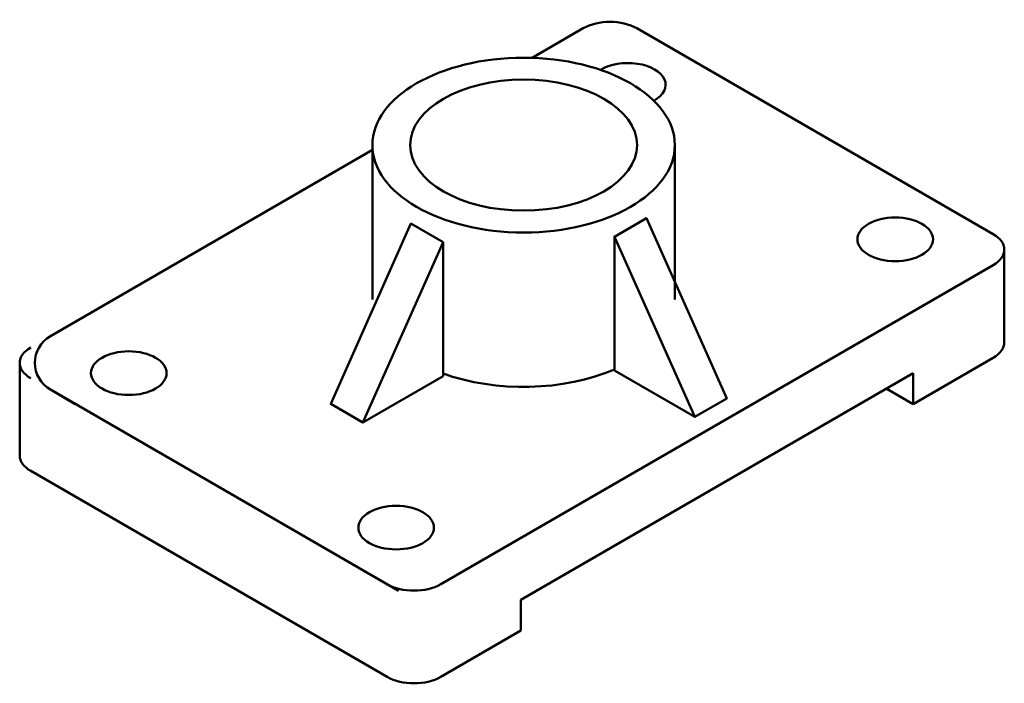
# Model space of a CAD drawing. Units: millimetres. Extents: x 2166 to 2644, y 1138 to 1460.
import ezdxf

# ---------------------------------------------------------------- set-up
doc = ezdxf.new("R2010")
doc.units = ezdxf.units.MM
doc.layers.add('M-OUTL', color=7, linetype='Continuous', lineweight=50)

msp = doc.modelspace()

# ---------------------------------------------------------------- linework, layer by layer
at = {"layer": 'M-OUTL'}
for p, q in [((2414.45, 1441.4), (2439.37, 1455.79)), ((2638.56, 1355.79), (2465.35, 1455.79)), ((2336.87, 1399.04), (2336.87, 1324.04)), ((2483.84, 1399.04), (2483.84, 1324.04)), ((2643.94, 1303.29), (2643.94, 1348.29)), ((2370.09, 1185.79), (2638.56, 1340.79)), ((2165.52, 1248.29), (2165.52, 1293.29)), ((2599.58, 1273.29), (2638.56, 1295.79)), ((2409.06, 1178.29), (2599.58, 1288.29)), ((2599.58, 1273.29), (2599.58, 1288.29)), ((2180.41, 1280.3), (2349.6, 1182.62)), ((2599.58, 1273.29), (2586.59, 1280.79)), ((2344.11, 1140.79), (2170.9, 1240.79)), ((2409.06, 1163.29), (2409.06, 1178.29)), ((2370.09, 1140.79), (2409.06, 1163.29))]:
    msp.add_line(p, q, dxfattribs=at)
msp.add_lwpolyline([(2336.98, 1396.68), (2180.41, 1306.28, 0.57735), (2180.41, 1280.3), (2192.55, 1273.29)], format="xyb", dxfattribs=at)
for points in [[(2493.49, 1267.04), (2509.08, 1276.04), (2470.11, 1363.54), (2454.52, 1354.54)], [(2332.25, 1264.39), (2316.66, 1273.39), (2355.63, 1360.89), (2371.22, 1351.89)]]:
    msp.add_lwpolyline(points, dxfattribs=at)
for points in [[(2454.52, 1289.54), (2493.49, 1267.04), (2454.52, 1354.54)], [(2371.22, 1286.89), (2332.25, 1264.39), (2371.22, 1351.89)]]:
    msp.add_lwpolyline(points, close=True, dxfattribs=at)
for centre, major_axis, start_param, end_param in [((2452.36, 1448.29), (-18.37, 0), 3.926991, 5.497787), ((2461.02, 1428.29), (-18.37, 0), 2.32895, 5.525032), ((2625.57, 1348.29), (18.37, 0), 0, 0.785398), ((2625.57, 1348.29), (18.37, 0), 5.497787, 6.283185), ((2625.57, 1303.29), (18.37, 0), 5.497787, 6.283185), ((2183.89, 1293.29), (-18.37, 0), 5.497787, 6.283185), ((2183.89, 1293.29), (-18.37, 0), 0, 0.785398), ((2410.36, 1324.04), (73.48, 0), 4.146433, 5.357192), ((2183.89, 1248.29), (-18.37, 0), 0, 0.785398), ((2357.1, 1193.29), (18.37, 0), 3.926991, 5.497787), ((2357.1, 1148.29), (18.37, 0), 3.926991, 5.497787)]:
    msp.add_ellipse(centre, major_axis=major_axis, ratio=0.57735, start_param=start_param, end_param=end_param, dxfattribs=at)
for centre, major_axis in [((2410.36, 1399.04), (-73.48, 0)), ((2410.36, 1399.04), (-55.11, 0)), ((2590.93, 1353.29), (-18.37, 0)), ((2218.53, 1288.29), (-18.37, 0)), ((2348.44, 1213.29), (-18.37, 0))]:
    msp.add_ellipse(centre, major_axis=major_axis, ratio=0.57735, dxfattribs=at)

doc.saveas('drawing.dxf')
